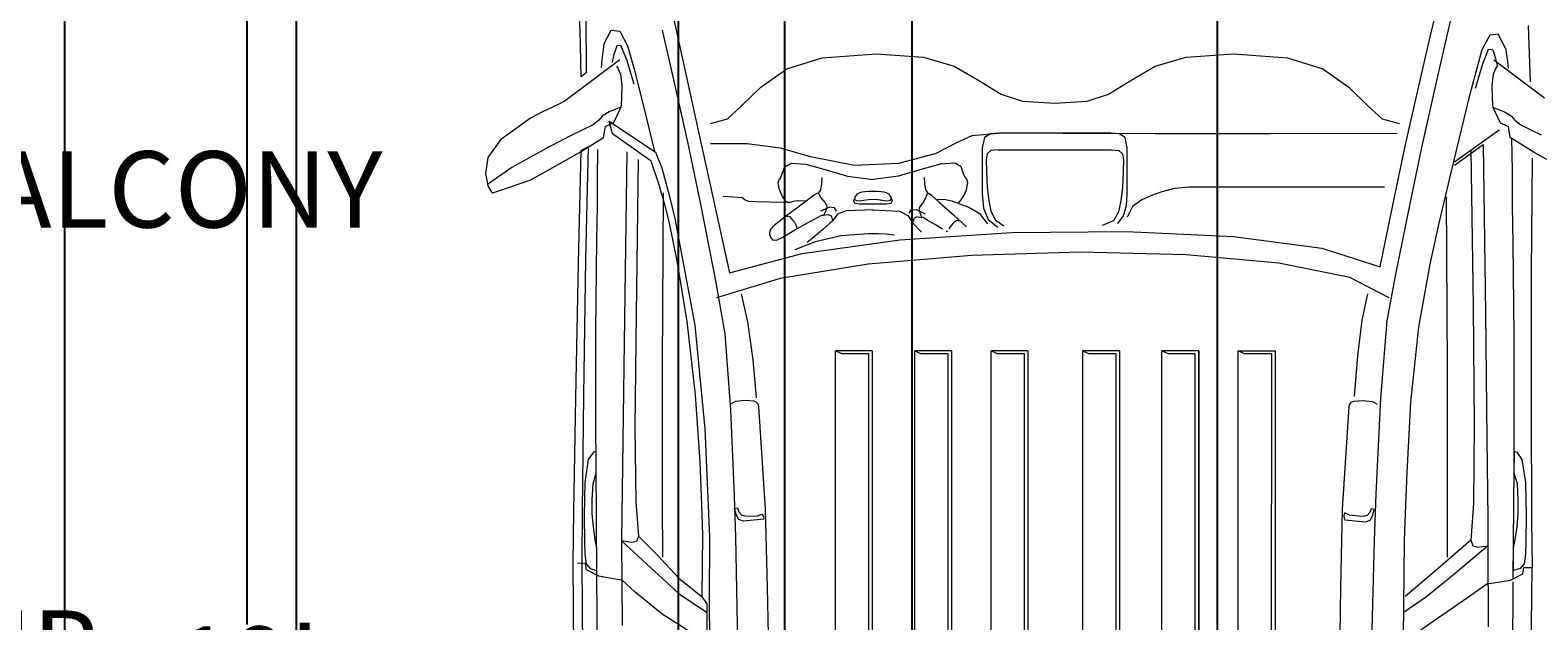
# Model space of a CAD drawing. Units: inches. Extents: x -36 to 401, y -686 to 73.
# Tile 5 of 15: x 184 to 303, y -532 to -485. Entities that reach past the tile are written whole.
import ezdxf

# ---------------------------------------------------------------- set-up
doc = ezdxf.new("R2010")
doc.units = ezdxf.units.IN
doc.header["$MEASUREMENT"] = 0
for name, color, linetype, lineweight in [('A-ANNO-DIMS', 2, 'Continuous', 18), ('A-ANNO-TEXT', 7, 'Continuous', 18), ('A-AREA-IDEN', 7, 'Continuous', 18), ('C-PKNG-VEHI', 8, 'Continuous', 13)]:
    doc.layers.add(name, color=color, linetype=linetype, lineweight=lineweight)
doc.styles.get("Standard").update_dxf_attribs({"font": 'arial.ttf'})
doc.dimstyles.get("Standard").update_dxf_attribs({"dimtxt": 0.18, "dimasz": 0.18, "dimexe": 0.18, "dimexo": 0.0625, "dimgap": 0.09, "dimtad": 0, "dimtih": 1, "dimtoh": 1, "dimdec": 0, "dimzin": 0, "dimdsep": 46, "dimlunit": 3, "dimtxsty": 'Standard', "dimcen": 0.09, "dimadec": 0, "dimazin": 0, "dimtfac": 1, "dimtdec": 0, "dimtofl": 0, "dimtmove": 0, "dimatfit": 3, "dimfxl": 1, "dimtolj": 1, "dimtzin": 0, "dimarcsym": 0})

# ---------------------------------------------------------------- blocks, each defined once
blk = doc.blocks.new('*D3')
at = {"layer": 'A-ANNO-DIMS', "color": 0, "lineweight": -2, "transparency": 16777216}
for p, q in [((200.9, -421.21), (201.62, -421.21)), ((201.44, -421.39), (201.44, -532.06)), ((201.44, -649.03), (201.44, -538.36)), ((200.9, -649.21), (201.62, -649.21))]:
    blk.add_line(p, q, dxfattribs=at)
at = {"layer": 'A-ANNO-DIMS', "color": 0, "transparency": 16777216}
for points in [[(201.41, -421.39), (201.47, -421.39), (201.44, -421.21)], [(201.41, -649.03), (201.47, -649.03), (201.44, -649.21)]]:
    blk.add_solid(points, dxfattribs=at)
at = {"layer": 'Defpoints', "color": 0, "transparency": 16777216}
for p in [(200.84, -421.21), (200.84, -649.21), (201.44, -649.21)]:
    blk.add_point(p, dxfattribs=at)
at = {"layer": 'A-ANNO-DIMS', "color": 0, "transparency": 16777216, "insert": (201.44, -535.21), "char_height": 6, "attachment_point": 5}
blk.add_mtext("\\A1;19'", dxfattribs=at)
blk = doc.blocks.new('*D73')
at = {"layer": 'A-ANNO-DIMS', "color": 0, "lineweight": -2, "transparency": 16777216}
for p, q in [((177.19, -421.27), (177.19, -685.69)), ((253.69, -421.27), (253.69, -685.69)), ((177.37, -685.51), (214.9, -685.51)), ((253.51, -685.51), (215.98, -685.51))]:
    blk.add_line(p, q, dxfattribs=at)
at = {"layer": 'A-ANNO-DIMS', "color": 0, "transparency": 16777216}
for points in [[(177.37, -685.48), (177.37, -685.54), (177.19, -685.51)], [(253.51, -685.48), (253.51, -685.54), (253.69, -685.51)]]:
    blk.add_solid(points, dxfattribs=at)
at = {"layer": 'Defpoints', "color": 0, "transparency": 16777216}
for p in [(177.19, -421.21), (253.69, -421.21), (253.69, -685.51)]:
    blk.add_point(p, dxfattribs=at)
at = {"layer": 'A-ANNO-DIMS', "color": 0, "transparency": 16777216, "insert": (215.44, -685.51), "char_height": 0.18, "attachment_point": 5}
blk.add_mtext('\\A1;6\'-4 1/2"', dxfattribs=at)
blk = doc.blocks.new('*D74')
at = {"layer": 'A-ANNO-DIMS', "color": 0, "lineweight": -2, "transparency": 16777216}
for p, q in [((277.69, -412.27), (277.69, -685.69)), ((313.69, -421.27), (313.69, -685.69)), ((277.87, -685.51), (295.36, -685.51)), ((313.51, -685.51), (296.02, -685.51))]:
    blk.add_line(p, q, dxfattribs=at)
at = {"layer": 'A-ANNO-DIMS', "color": 0, "transparency": 16777216}
for points in [[(277.87, -685.48), (277.87, -685.54), (277.69, -685.51)], [(313.51, -685.48), (313.51, -685.54), (313.69, -685.51)]]:
    blk.add_solid(points, dxfattribs=at)
at = {"layer": 'Defpoints', "color": 0, "transparency": 16777216}
for p in [(277.69, -412.21), (313.69, -421.21), (313.69, -685.51)]:
    blk.add_point(p, dxfattribs=at)
at = {"layer": 'A-ANNO-DIMS', "color": 0, "transparency": 16777216, "insert": (295.69, -685.51), "char_height": 0.18, "attachment_point": 5}
blk.add_mtext('\\A1;3\'-0"', dxfattribs=at)
blk = doc.blocks.new('*D87')
at = {"layer": 'A-ANNO-DIMS', "color": 0, "lineweight": -2, "transparency": 16777216}
for p, q in [((243.7, -154.81), (243.7, -685.69)), ((187.11, -163.6), (187.11, -685.69)), ((187.29, -685.51), (214.86, -685.51)), ((243.52, -685.51), (215.95, -685.51))]:
    blk.add_line(p, q, dxfattribs=at)
at = {"layer": 'A-ANNO-DIMS', "color": 0, "transparency": 16777216}
for points in [[(187.29, -685.48), (187.29, -685.54), (187.11, -685.51)], [(243.52, -685.48), (243.52, -685.54), (243.7, -685.51)]]:
    blk.add_solid(points, dxfattribs=at)
at = {"layer": 'Defpoints', "color": 0, "transparency": 16777216}
for p in [(243.7, -154.75), (187.11, -163.53), (243.7, -685.51)]:
    blk.add_point(p, dxfattribs=at)
at = {"layer": 'A-ANNO-DIMS', "color": 0, "transparency": 16777216, "insert": (215.4, -685.51), "char_height": 0.18, "attachment_point": 5}
blk.add_mtext('\\A1;4\'-8 1/2"', dxfattribs=at)
blk = doc.blocks.new('*D91')
at = {"layer": 'A-ANNO-DIMS', "color": 0, "lineweight": -2, "transparency": 16777216}
for p, q in [((205.32, -404.21), (205.32, -685.69)), ((235.34, -404.21), (235.34, -685.69)), ((205.5, -685.51), (220, -685.51)), ((235.16, -685.51), (220.66, -685.51))]:
    blk.add_line(p, q, dxfattribs=at)
at = {"layer": 'A-ANNO-DIMS', "color": 0, "transparency": 16777216}
for points in [[(205.5, -685.48), (205.5, -685.54), (205.32, -685.51)], [(235.16, -685.48), (235.16, -685.54), (235.34, -685.51)]]:
    blk.add_solid(points, dxfattribs=at)
at = {"layer": 'Defpoints', "color": 0, "transparency": 16777216}
for p in [(205.32, -404.14), (235.34, -404.14), (235.34, -685.51)]:
    blk.add_point(p, dxfattribs=at)
at = {"layer": 'A-ANNO-DIMS', "color": 0, "transparency": 16777216, "insert": (220.33, -685.51), "char_height": 0.18, "attachment_point": 5}
blk.add_mtext('\\A1;2\'-6"', dxfattribs=at)

msp = doc.modelspace()

# ---------------------------------------------------------------- linework, layer by layer
at = {"layer": 'C-PKNG-VEHI'}
for p, q in [((227.62, -485.32), (227.51, -482.83)), ((296.28, -483.48), (295.79, -485.61)), ((228.07, -484.2), (228.11, -488.65)), ((234.84, -483.75), (239.36, -504.4)), ((294.45, -485.83), (294.91, -483.89)), ((227.72, -488.98), (227.62, -485.32)), ((229.5, -486.4), (230.08, -485.31)), ((230.08, -485.31), (230.74, -485.39)), ((230.74, -485.39), (231.36, -486.54)), ((234.08, -485.3), (235.13, -489.89)), ((293.47, -490.06), (294.45, -485.83)), ((295.79, -485.61), (294.73, -490.2)), ((299.13, -485.7), (298.5, -486.85)), ((299.79, -485.61), (299.13, -485.7)), ((300.37, -486.71), (299.79, -485.61)), ((302.16, -484.94), (302.3, -489.38)), ((229.41, -487.01), (229.33, -487.64)), ((229.5, -486.4), (229.41, -487.01)), ((230.5, -486.54), (230.28, -487.23)), ((230.84, -486.5), (230.5, -486.54)), ((231.29, -487.65), (230.84, -486.5)), ((231.36, -486.54), (231.88, -488.37)), ((298.5, -486.85), (297.48, -490.66)), ((298.58, -487.95), (299.03, -486.8)), ((299.03, -486.8), (299.36, -486.85)), ((299.36, -486.85), (299.59, -487.54)), ((300.37, -486.71), (300.45, -487.24)), ((230.76, -487.64), (228.02, -489.69)), ((229.33, -487.64), (229.27, -488.27)), ((230.17, -487.68), (230.14, -487.84)), ((230.28, -487.23), (230.17, -487.68)), ((230.48, -488.14), (230.59, -488.3)), ((231.87, -489.56), (231.29, -487.65)), ((243.88, -488.35), (246.64, -487.47)), ((246.64, -487.47), (250.89, -487.17)), ((250.89, -487.17), (254.61, -487.42)), ((254.61, -487.42), (257.04, -488.14)), ((257.04, -488.14), (259.01, -489.28)), ((270.87, -489.28), (272.84, -488.14)), ((272.84, -488.14), (275.27, -487.42)), ((275.27, -487.42), (278.99, -487.17)), ((278.99, -487.17), (283.24, -487.47)), ((283.24, -487.47), (286, -488.35)), ((298, -489.87), (298.58, -487.95)), ((299.44, -487.64), (302.18, -489.69)), ((299.59, -487.54), (299.69, -487.98)), ((299.72, -488.14), (299.61, -488.3)), ((299.69, -487.98), (299.72, -488.14)), ((300.45, -487.24), (300.51, -487.78)), ((300.51, -487.78), (300.57, -488.33)), ((228.11, -488.65), (227.72, -488.98)), ((230.59, -488.3), (230.79, -488.78)), ((230.79, -488.78), (230.91, -489.65)), ((231.88, -488.37), (232.64, -491.39)), ((241.82, -489.78), (243.88, -488.35)), ((259.01, -489.28), (260.72, -490.33)), ((269.16, -490.33), (270.87, -489.28)), ((286, -488.35), (288.06, -489.78)), ((299.4, -488.78), (299.29, -489.65)), ((299.61, -488.3), (299.4, -488.78)), ((228.02, -489.69), (226.76, -490.64)), ((230.89, -490.58), (230.85, -491.17)), ((230.91, -489.65), (230.89, -490.58)), ((235.13, -489.89), (236.1, -494.23)), ((240.29, -491.28), (241.82, -489.78)), ((260.72, -490.33), (262.39, -490.89)), ((267.49, -490.89), (269.16, -490.33)), ((288.06, -489.78), (289.58, -491.28)), ((292.54, -494.2), (293.47, -490.06)), ((294.73, -490.2), (293.76, -494.53)), ((299.29, -489.65), (299.31, -490.58)), ((299.31, -490.58), (299.35, -491.17)), ((302.18, -489.69), (303.44, -490.64)), ((224.63, -491.76), (223.73, -492.24)), ((225.85, -491.17), (224.63, -491.76)), ((226.45, -490.87), (225.85, -491.17)), ((226.76, -490.64), (226.45, -490.87)), ((229.91, -491.73), (229.37, -492.07)), ((230.83, -491.37), (229.91, -491.73)), ((230.83, -491.37), (230.26, -492.6)), ((230.85, -491.17), (230.83, -491.37)), ((232.64, -491.39), (233.47, -494.86)), ((239.2, -492.29), (240.29, -491.28)), ((262.39, -490.89), (264.94, -491.05)), ((264.94, -491.05), (267.49, -490.89)), ((289.58, -491.28), (290.68, -492.29)), ((297.48, -490.66), (296.1, -496.4)), ((299.35, -491.17), (299.36, -491.37)), ((299.36, -491.37), (299.94, -492.6)), ((299.36, -491.37), (300.29, -491.73)), ((300.29, -491.73), (300.83, -492.07)), ((223.73, -492.24), (221.36, -493.94)), ((228.64, -492.74), (227.79, -493.17)), ((229.11, -492.38), (228.64, -492.74)), ((229.37, -492.07), (229.11, -492.38)), ((229.47, -493.74), (229.61, -492.88)), ((230.26, -492.6), (229.61, -492.88)), ((229.92, -492.46), (233.56, -494.9)), ((230.17, -493.46), (229.92, -492.46)), ((237.87, -492.64), (239.2, -492.29)), ((290.68, -492.29), (292.01, -492.64)), ((299.94, -492.6), (300.59, -492.88)), ((300.73, -493.74), (300.59, -492.88)), ((300.83, -492.07), (301.09, -492.38)), ((301.09, -492.38), (301.56, -492.74)), ((301.56, -492.74), (302.41, -493.17)), ((221.36, -493.94), (220.36, -495.32)), ((227.03, -493.53), (225.2, -494.48)), ((227.79, -493.17), (227.03, -493.53)), ((227.58, -494.92), (229.47, -493.74)), ((233.22, -495.6), (230.17, -493.46)), ((257.21, -494.18), (255.53, -495.04)), ((258.43, -493.61), (257.21, -494.18)), ((260.81, -493.41), (258.43, -493.61)), ((259.41, -493.74), (259.23, -494.56)), ((259.88, -493.45), (259.41, -493.74)), ((260.53, -493.42), (259.88, -493.45)), ((269.35, -493.42), (260.53, -493.42)), ((265.59, -493.44), (260.81, -493.41)), ((272.84, -493.45), (265.59, -493.44)), ((270, -493.45), (269.35, -493.42)), ((270.47, -493.74), (270, -493.45)), ((270.64, -494.56), (270.47, -493.74)), ((281.84, -493.45), (272.84, -493.45)), ((291.84, -493.43), (281.84, -493.45)), ((299.87, -493.17), (296.35, -495.68)), ((302.62, -494.92), (300.73, -493.74)), ((300.85, -493.78), (300.88, -496.4)), ((302.41, -493.17), (303.17, -493.53)), ((220.36, -495.32), (220.2, -496.59)), ((225.2, -494.48), (222.27, -496.12)), ((223.76, -497.07), (227.58, -494.92)), ((227.49, -503.64), (227.72, -494.76)), ((227.72, -494.76), (228.25, -494.45)), ((228.25, -494.45), (228.04, -503.37)), ((228.99, -494.7), (228.97, -497)), ((231.3, -494.88), (231.12, -507.99)), ((233.56, -494.9), (234.05, -496.14)), ((236.1, -494.23), (237.12, -499.13)), ((240.75, -494.26), (237.87, -494.26)), ((243.38, -494.6), (240.75, -494.26)), ((245.74, -495.26), (243.38, -494.6)), ((249.19, -495.96), (245.74, -495.26)), ((255.53, -495.04), (252.65, -495.79)), ((259.23, -494.56), (259.23, -498.18)), ((259.62, -495.04), (259.55, -495.5)), ((259.91, -494.78), (259.62, -495.04)), ((260.49, -494.71), (259.91, -494.78)), ((260.49, -494.71), (269.39, -494.71)), ((269.39, -494.71), (269.97, -494.78)), ((269.97, -494.78), (270.26, -495.04)), ((270.26, -495.04), (270.33, -495.5)), ((270.64, -498.18), (270.64, -494.56)), ((291.81, -497.67), (292.54, -494.2)), ((293.76, -494.53), (292.81, -499.1)), ((296.36, -495.93), (298.61, -494.3)), ((297.64, -494.75), (297.82, -507.04)), ((298.61, -494.3), (298.79, -507.56)), ((306.44, -497.07), (302.62, -494.92)), ((222.27, -496.12), (220.34, -497.45)), ((232.19, -495.49), (232.02, -507.62)), ((233.81, -497.39), (233.22, -495.6)), ((234.05, -496.14), (234.65, -498.4)), ((243.52, -496.61), (243.71, -496.05)), ((243.71, -496.05), (244.21, -495.76)), ((244.21, -495.76), (245.37, -495.84)), ((245.37, -495.84), (246.96, -496.28)), ((246.96, -496.28), (248.65, -496.8)), ((252.65, -495.79), (249.19, -495.96)), ((254.34, -496.28), (252.64, -496.8)), ((255.93, -495.84), (254.34, -496.28)), ((257.09, -495.76), (255.93, -495.84)), ((257.59, -496.05), (257.09, -495.76)), ((257.77, -496.61), (257.59, -496.05)), ((259.55, -495.5), (259.57, -496.42)), ((259.57, -496.42), (259.63, -497.65)), ((270.31, -496.42), (270.25, -497.65)), ((270.33, -495.5), (270.31, -496.42)), ((296.1, -496.4), (295.13, -500.49)), ((300.88, -496.4), (300.9, -499.16)), ((302.47, -495.38), (302.37, -504.35)), ((220.2, -496.59), (220.38, -497.56)), ((220.38, -497.56), (220.64, -498)), ((220.77, -498.1), (223.76, -497.07)), ((228.97, -497), (228.96, -499.15)), ((234.3, -499.12), (233.81, -497.39)), ((243.2, -497.31), (243.27, -497.02)), ((243.29, -497.87), (243.2, -497.31)), ((243.27, -497.02), (243.38, -496.96)), ((243.38, -496.96), (243.52, -496.61)), ((246.6, -497.39), (246.52, -497.86)), ((246.62, -496.89), (246.6, -497.39)), ((248.65, -496.8), (250.65, -497.05)), ((252.64, -496.8), (250.65, -497.05)), ((254.67, -496.89), (254.7, -497.38)), ((254.7, -497.38), (254.78, -497.86)), ((257.91, -496.96), (257.77, -496.61)), ((258.02, -497.02), (257.91, -496.96)), ((258, -497.87), (258.09, -497.31)), ((258.09, -497.31), (258.02, -497.02)), ((259.63, -497.65), (259.75, -498.74)), ((270.25, -497.65), (270.13, -498.74)), ((275.5, -497.66), (274.35, -497.77)), ((290.85, -497.66), (275.5, -497.66)), ((290.94, -501.87), (291.81, -497.67)), ((220.64, -498), (220.77, -498.1)), ((234.16, -498.1), (234.08, -511.66)), ((234.65, -498.4), (235.06, -500.11)), ((240.4, -498.49), (238.87, -498.38)), ((240.44, -498.55), (240.4, -498.49)), ((240.6, -498.67), (240.44, -498.55)), ((240.9, -498.77), (240.6, -498.67)), ((241.49, -498.81), (240.9, -498.77)), ((242.54, -498.84), (241.49, -498.81)), ((244.15, -498.85), (242.54, -498.84)), ((243.51, -498.34), (243.29, -497.87)), ((243.72, -498.66), (243.51, -498.34)), ((243.86, -498.82), (243.72, -498.66)), ((245.18, -498.92), (243.74, -499.98)), ((243.99, -498.88), (243.86, -498.82)), ((244.15, -498.85), (243.99, -498.88)), ((244.37, -498.77), (244.15, -498.85)), ((244.74, -498.73), (244.37, -498.77)), ((245.31, -498.75), (244.74, -498.73)), ((246.05, -498.27), (245.18, -498.92)), ((246.23, -498.16), (246.05, -498.27)), ((246.3, -498.16), (246.23, -498.16)), ((246.31, -498.18), (246.3, -498.16)), ((246.52, -497.86), (246.31, -498.18)), ((246.39, -498.18), (246.52, -498.46)), ((246.52, -498.46), (246.7, -498.69)), ((246.7, -498.69), (246.89, -498.89)), ((246.89, -498.89), (247, -499.08)), ((249.14, -498.74), (249.24, -498.44)), ((249.23, -498.93), (249.14, -498.74)), ((249.23, -498.59), (249.24, -498.44)), ((249.34, -498.73), (249.23, -498.59)), ((249.58, -498.99), (249.23, -498.93)), ((249.24, -498.44), (249.42, -498.19)), ((249.58, -498.75), (249.34, -498.73)), ((249.42, -498.19), (249.61, -498.08)), ((249.91, -498.7), (249.58, -498.75)), ((249.61, -498.08), (249.8, -498.03)), ((249.8, -498.03), (250.03, -498)), ((250.29, -498.65), (249.91, -498.7)), ((250.03, -498), (250.33, -497.98)), ((250.66, -498.62), (250.29, -498.65)), ((250.33, -497.98), (250.65, -497.98)), ((250.65, -497.98), (250.97, -497.98)), ((251.03, -498.65), (250.66, -498.62)), ((250.97, -497.98), (251.26, -498)), ((251.39, -498.7), (251.03, -498.65)), ((251.26, -498), (251.5, -498.03)), ((251.72, -498.75), (251.39, -498.7)), ((251.5, -498.03), (251.68, -498.08)), ((251.68, -498.08), (251.87, -498.19)), ((251.95, -498.73), (251.72, -498.75)), ((252.06, -498.93), (251.72, -498.99)), ((251.87, -498.19), (252.05, -498.44)), ((252.06, -498.59), (251.95, -498.73)), ((252.05, -498.44), (252.15, -498.74)), ((252.05, -498.44), (252.06, -498.59)), ((252.15, -498.74), (252.06, -498.93)), ((254.6, -498.84), (254.41, -499.09)), ((254.77, -498.51), (254.6, -498.84)), ((254.91, -498.18), (254.77, -498.51)), ((254.78, -497.86), (254.99, -498.18)), ((254.99, -498.18), (255, -498.16)), ((255, -498.16), (255.07, -498.16)), ((255.07, -498.16), (255.24, -498.29)), ((255.24, -498.29), (255.88, -498.85)), ((255.72, -498.61), (256.36, -498.62)), ((255.88, -498.85), (256.98, -499.84)), ((256.36, -498.62), (256.85, -498.73)), ((256.85, -498.73), (257.15, -498.85)), ((257.15, -498.85), (257.31, -498.88)), ((257.31, -498.88), (257.44, -498.82)), ((257.44, -498.82), (257.57, -498.66)), ((257.57, -498.66), (257.78, -498.34)), ((257.78, -498.34), (258, -497.87)), ((259.23, -498.18), (259.33, -499.3)), ((259.75, -498.74), (259.92, -499.51)), ((270.13, -498.74), (269.95, -499.59)), ((270.58, -499.11), (270.64, -498.18)), ((271.77, -498.66), (271.04, -499.18)), ((272.55, -498.32), (271.77, -498.66)), ((273.36, -498.03), (272.55, -498.32)), ((274.35, -497.77), (273.36, -498.03)), ((295.7, -498.41), (295.79, -511.89)), ((228.96, -499.15), (228.92, -501.77)), ((234.62, -500.35), (234.3, -499.12)), ((235.06, -500.11), (236.64, -508.5)), ((237.12, -499.13), (238.29, -505.15)), ((243.74, -499.98), (242.74, -500.78)), ((243.8, -499.97), (243.94, -499.93)), ((243.94, -499.93), (244.09, -499.97)), ((244.09, -499.97), (244.27, -500.16)), ((245.73, -500.32), (246.67, -499.84)), ((247.25, -499.22), (246.52, -499.54)), ((246.67, -499.84), (246.7, -499.85)), ((246.7, -499.85), (246.79, -499.86)), ((246.79, -499.86), (246.95, -499.84)), ((246.85, -499.68), (246.82, -499.79)), ((246.82, -499.79), (246.82, -499.83)), ((246.93, -499.48), (246.85, -499.68)), ((247.01, -499.27), (246.93, -499.48)), ((246.95, -499.84), (247.16, -499.81)), ((247, -499.08), (247.01, -499.27)), ((247.16, -499.81), (247.36, -499.92)), ((247.63, -499.27), (247.25, -499.22)), ((247.36, -499.92), (247.48, -500.27)), ((247.87, -499.78), (247.48, -500.27)), ((247.78, -499.55), (247.63, -499.27)), ((248.55, -499.52), (247.87, -499.78)), ((250.7, -499.44), (248.55, -499.52)), ((251.72, -498.99), (249.58, -498.99)), ((250.59, -499.44), (252.73, -499.55)), ((252.73, -499.55), (253.39, -499.89)), ((253.39, -499.89), (253.75, -500.43)), ((253.49, -499.7), (253.65, -499.43)), ((253.65, -499.43), (254.03, -499.4)), ((253.89, -500.09), (253.75, -500.43)), ((254.09, -499.99), (253.89, -500.09)), ((254.03, -499.4), (254.75, -499.75)), ((254.3, -500.03), (254.09, -499.99)), ((254.29, -499.27), (254.27, -499.46)), ((254.27, -499.46), (254.34, -499.68)), ((254.41, -499.09), (254.29, -499.27)), ((254.46, -500.06), (254.3, -500.03)), ((254.34, -499.68), (254.41, -499.87)), ((254.41, -499.87), (254.43, -499.99)), ((254.43, -499.99), (254.43, -500.03)), ((254.55, -500.05), (254.46, -500.06)), ((254.58, -500.05), (254.55, -500.05)), ((254.97, -500.27), (254.58, -500.05)), ((256.98, -499.84), (257.99, -500.77)), ((257.36, -498.93), (258.17, -499.23)), ((258.17, -499.23), (258.99, -499.7)), ((258.99, -499.7), (259.64, -500.55)), ((259.33, -499.3), (259.7, -500.21)), ((259.92, -499.51), (260.25, -500.22)), ((269.95, -499.59), (269.55, -500.31)), ((269.89, -500.51), (270.35, -499.9)), ((270.35, -499.9), (270.58, -499.11)), ((271.04, -499.18), (270.63, -500.02)), ((292.81, -499.1), (291.73, -504.49)), ((300.9, -499.16), (300.94, -502.07)), ((235.26, -503.46), (234.62, -500.35)), ((242.54, -501.07), (242.5, -501.35)), ((242.74, -500.78), (242.54, -501.07)), ((243.57, -501.58), (244.51, -501)), ((244.27, -500.16), (244.47, -500.42)), ((244.47, -500.42), (244.62, -500.67)), ((244.51, -501), (245.73, -500.32)), ((244.62, -500.67), (244.66, -500.9)), ((246.68, -501), (245.86, -501.7)), ((247.48, -500.27), (246.68, -501)), ((252.77, -501.81), (261.55, -501.23)), ((253.75, -500.43), (253.96, -500.67)), ((253.96, -500.67), (254.19, -500.92)), ((254.19, -500.92), (254.45, -501.2)), ((255.5, -500.58), (254.97, -500.27)), ((256.11, -500.96), (255.5, -500.58)), ((256.41, -501.13), (256.51, -501.12)), ((256.44, -501.13), (256.41, -501.13)), ((256.48, -501.13), (256.44, -501.13)), ((256.51, -501.12), (256.48, -501.13)), ((256.7, -500.8), (256.6, -500.95)), ((256.82, -500.65), (256.7, -500.8)), ((256.96, -500.49), (256.82, -500.65)), ((257.15, -500.32), (256.96, -500.49)), ((257.3, -500.28), (257.15, -500.32)), ((257.44, -500.32), (257.3, -500.28)), ((259.7, -500.21), (260.46, -500.81)), ((260.25, -500.22), (260.93, -500.69)), ((261.55, -501.23), (270.57, -501.13)), ((269.55, -500.31), (268.65, -500.68)), ((270.57, -501.13), (278.98, -501.54)), ((295.13, -500.49), (294.41, -503.71)), ((228.92, -501.77), (228.84, -509.04)), ((242.5, -501.35), (242.58, -501.6)), ((242.58, -501.6), (242.76, -501.8)), ((242.76, -501.8), (243.07, -501.83)), ((243.07, -501.83), (243.57, -501.58)), ((244.52, -502.57), (246.13, -501.93)), ((245.09, -502.87), (252.77, -501.81)), ((245.86, -501.7), (245.48, -502.02)), ((246.13, -501.93), (248.12, -501.47)), ((248.12, -501.47), (250.33, -501.3)), ((250.33, -501.3), (251.05, -501.3)), ((251.05, -501.3), (251.68, -501.33)), ((251.68, -501.33), (252.34, -501.41)), ((278.98, -501.54), (285.92, -502.46)), ((285.92, -502.46), (290.52, -503.91)), ((290.52, -503.91), (290.94, -501.87)), ((300.94, -502.07), (301.03, -509.35)), ((227.28, -514.2), (227.49, -503.64)), ((228.04, -503.37), (227.88, -514.04)), ((236.03, -508.21), (235.26, -503.46)), ((239.36, -504.4), (245.09, -502.87)), ((258.38, -503.03), (250.27, -503.71)), ((266.96, -502.78), (258.38, -503.03)), ((275.26, -502.98), (266.96, -502.78)), ((282.56, -503.63), (275.26, -502.98)), ((288.12, -504.75), (282.56, -503.63)), ((243.35, -504.83), (238.35, -506.35)), ((250.27, -503.71), (243.35, -504.83)), ((291.22, -506.35), (288.12, -504.75)), ((291.73, -504.49), (291.05, -508.18)), ((294.41, -503.71), (293.53, -508.67)), ((302.37, -504.35), (302.38, -514.97)), ((238.29, -505.15), (238.99, -509.18)), ((240.29, -506.05), (240.78, -508.26)), ((289.53, -506.05), (289.07, -508.12)), ((297.82, -507.04), (297.91, -516.35)), ((231.12, -507.99), (230.99, -517.58)), ((232.02, -507.62), (231.94, -516.57)), ((236.7, -513.98), (236.03, -508.21)), ((240.78, -508.26), (241.19, -511.23)), ((289.07, -508.12), (288.72, -510.92)), ((291.05, -508.18), (290.54, -514.26)), ((298.79, -507.56), (298.91, -517.49)), ((228.84, -509.04), (228.84, -516.24)), ((236.64, -508.5), (237.44, -516.67)), ((238.99, -509.18), (239.44, -515.16)), ((293.53, -508.67), (292.9, -514.57)), ((301.03, -509.35), (301.03, -516.55)), ((247.7, -586.39), (247.7, -510.52)), ((248.19, -510.76), (247.7, -510.52)), ((250.59, -510.52), (247.7, -510.52)), ((250.33, -510.76), (248.19, -510.76)), ((250.3, -585.18), (250.33, -510.76)), ((250.59, -510.52), (250.59, -586.39)), ((250.59, -510.52), (250.59, -586.39)), ((253.93, -586.39), (253.93, -510.52)), ((254.42, -510.76), (253.93, -510.52)), ((256.82, -510.52), (253.93, -510.52)), ((256.56, -510.76), (254.42, -510.76)), ((256.53, -585.18), (256.56, -510.76)), ((256.82, -510.52), (256.82, -586.39)), ((256.82, -510.52), (256.82, -586.39)), ((259.94, -586.39), (259.94, -510.52)), ((260.43, -510.76), (259.94, -510.52)), ((262.83, -510.52), (259.94, -510.52)), ((262.57, -510.76), (260.43, -510.76)), ((262.54, -585.18), (262.57, -510.76)), ((262.83, -510.52), (262.83, -586.39)), ((262.83, -510.52), (262.83, -586.39)), ((267.61, -510.76), (267.12, -510.52)), ((270.02, -510.52), (267.12, -510.52)), ((267.13, -586.39), (267.13, -510.52)), ((269.76, -510.76), (267.61, -510.76)), ((269.73, -585.18), (269.76, -510.76)), ((270.02, -510.52), (270.02, -586.39)), ((270.02, -510.52), (270.02, -586.39)), ((273.84, -510.76), (273.35, -510.52)), ((276.25, -510.52), (273.35, -510.52)), ((273.36, -586.39), (273.36, -510.52)), ((275.98, -510.76), (273.84, -510.76)), ((275.96, -585.18), (275.98, -510.76)), ((276.24, -510.52), (276.24, -586.39)), ((276.25, -510.52), (276.25, -586.39)), ((279.36, -586.39), (279.36, -510.52)), ((279.85, -510.76), (279.36, -510.52)), ((279.36, -510.52), (282.25, -510.52)), ((281.99, -510.76), (279.85, -510.76)), ((281.97, -585.18), (281.99, -510.76)), ((282.25, -510.52), (282.25, -586.39)), ((234.08, -511.66), (234.07, -522.4)), ((241.19, -511.23), (241.46, -514.23)), ((288.72, -510.92), (288.46, -514.12)), ((295.79, -511.89), (295.79, -522.48)), ((227.14, -523.17), (227.28, -514.2)), ((227.88, -514.04), (227.78, -523.12)), ((237.06, -519.26), (236.7, -513.98)), ((290.54, -514.26), (290.17, -521.79)), ((239.44, -515.16), (239.73, -521.94)), ((239.85, -514.51), (239.45, -514.73)), ((240.61, -514.43), (239.85, -514.51)), ((241.3, -514.49), (240.61, -514.43)), ((241.47, -514.58), (241.3, -514.49)), ((241.62, -514.72), (241.47, -514.58)), ((241.68, -514.9), (241.62, -514.72)), ((242.2, -522.99), (241.68, -514.9)), ((287.56, -522.99), (288.07, -514.9)), ((288.07, -514.9), (288.13, -514.72)), ((288.13, -514.72), (288.27, -514.58)), ((288.27, -514.58), (288.45, -514.49)), ((288.45, -514.49), (289.13, -514.43)), ((289.13, -514.43), (289.9, -514.51)), ((289.9, -514.51), (290.29, -514.73)), ((292.9, -514.57), (292.61, -520.11)), ((302.38, -514.97), (302.42, -523.85)), ((228.84, -516.24), (228.85, -519.5)), ((231.94, -516.57), (232, -522.38)), ((237.44, -516.67), (237.8, -525.17)), ((297.91, -516.35), (297.86, -522.53)), ((301.03, -516.55), (301.02, -519.81)), ((230.99, -517.58), (230.91, -523.46)), ((298.91, -517.49), (298.97, -523.71)), ((228.67, -518.5), (228.27, -519.08)), ((228.88, -518.46), (228.67, -518.5)), ((228.9, -520.15), (228.88, -518.46)), ((301.04, -520.15), (301.06, -518.46)), ((301.06, -518.46), (301.26, -518.5)), ((301.26, -518.5), (301.66, -519.08)), ((228.27, -519.08), (227.99, -520.89)), ((228.64, -520.98), (228.9, -520.15)), ((228.85, -519.5), (228.92, -528.19)), ((237.22, -523.35), (237.06, -519.26)), ((292.61, -520.11), (292.45, -524.01)), ((301.02, -519.81), (300.94, -528.5)), ((301.3, -520.98), (301.04, -520.15)), ((301.66, -519.08), (301.94, -520.89)), ((227.99, -520.89), (227.94, -523.48)), ((228.57, -522.21), (228.64, -520.98)), ((301.37, -522.21), (301.3, -520.98)), ((301.94, -520.89), (301.99, -523.48)), ((228.57, -523.32), (228.57, -522.21)), ((232, -522.38), (232.22, -525.1)), ((234.07, -522.4), (234.09, -526.77)), ((239.73, -521.94), (239.84, -525.17)), ((290.17, -521.79), (290.03, -525.48)), ((295.79, -522.48), (295.77, -526.77)), ((297.86, -522.53), (297.64, -525.41)), ((301.36, -523.32), (301.37, -522.21)), ((227.08, -527.24), (227.14, -523.17)), ((227.78, -523.12), (227.75, -527.24)), ((227.94, -523.48), (227.97, -525.61)), ((228.67, -524.41), (228.57, -523.32)), ((230.91, -523.46), (230.89, -525.47)), ((237.26, -524.99), (237.22, -523.35)), ((239.76, -522.94), (240.01, -522.89)), ((239.88, -523.4), (239.76, -522.94)), ((240.09, -523.79), (239.88, -523.4)), ((240.01, -522.89), (240.11, -523.19)), ((240.47, -523.93), (240.09, -523.79)), ((240.11, -523.19), (240.31, -523.43)), ((240.31, -523.43), (240.61, -523.51)), ((242.08, -523.77), (240.47, -523.93)), ((240.61, -523.51), (240.95, -523.53)), ((240.95, -523.53), (241.58, -523.52)), ((241.58, -523.52), (241.92, -523.37)), ((241.92, -523.37), (242.04, -523.56)), ((242.04, -523.56), (242.08, -523.71)), ((242.08, -523.71), (242.08, -523.77)), ((242.36, -529.15), (242.2, -522.99)), ((287.43, -529.15), (287.56, -522.99)), ((287.73, -523.26), (287.65, -523.49)), ((287.65, -523.49), (287.69, -523.72)), ((287.69, -523.72), (287.73, -523.82)), ((288.11, -523.45), (287.73, -523.26)), ((288.82, -523.54), (288.11, -523.45)), ((289.2, -523.57), (288.82, -523.54)), ((289.5, -523.49), (289.2, -523.57)), ((289.7, -523.24), (289.5, -523.49)), ((289.8, -522.95), (289.7, -523.24)), ((289.72, -523.85), (289.94, -523.46)), ((290.05, -523), (289.8, -522.95)), ((289.94, -523.46), (290.05, -523)), ((298.97, -523.71), (298.98, -525.86)), ((301.27, -524.41), (301.36, -523.32)), ((301.99, -523.48), (301.97, -525.61)), ((228.84, -525.52), (228.67, -524.41)), ((237.21, -529.88), (237.26, -524.99)), ((287.73, -523.82), (289.35, -523.98)), ((289.35, -523.98), (289.72, -523.85)), ((292.45, -524.01), (292.4, -525.48)), ((301.1, -525.52), (301.27, -524.41)), ((302.42, -523.85), (302.45, -527.56)), ((227.97, -525.61), (228, -526.5)), ((228.93, -526.04), (228.84, -525.52)), ((228.93, -527.8), (228.93, -526.04)), ((230.89, -525.47), (233.15, -527.56)), ((231.67, -525.61), (230.89, -525.47)), ((230.89, -525.47), (230.92, -532.14)), ((232.07, -525.53), (231.67, -525.61)), ((232.22, -525.1), (232.07, -525.53)), ((232.22, -525.1), (233.66, -526.54)), ((237.8, -525.17), (237.77, -530.16)), ((239.84, -525.17), (240, -533.51)), ((290.03, -525.48), (289.82, -533.45)), ((292.4, -525.48), (292.33, -533.09)), ((297.64, -525.41), (295.26, -527.5)), ((298.98, -525.86), (296.56, -527.92)), ((297.64, -525.41), (297.8, -525.86)), ((297.8, -525.86), (298.2, -525.98)), ((298.2, -525.98), (298.98, -525.86)), ((298.98, -525.86), (299.01, -532.23)), ((301, -526.04), (301.1, -525.52)), ((301, -527.8), (301, -526.04)), ((301.97, -525.61), (301.94, -526.5)), ((227.14, -534.09), (227.08, -527.24)), ((228.06, -527.26), (227.41, -527.24)), ((227.75, -527.24), (227.81, -534.08)), ((228, -526.5), (228.11, -527.28)), ((228.13, -527.76), (228.06, -527.26)), ((228.11, -527.28), (228.41, -527.66)), ((233.66, -526.54), (235.41, -528.43)), ((301.83, -527.28), (301.53, -527.66)), ((301.94, -526.5), (301.83, -527.28)), ((229.09, -528.26), (228.13, -527.76)), ((228.41, -527.66), (228.93, -527.8)), ((228.92, -528.19), (228.98, -538.68)), ((230.24, -528.46), (229.09, -528.26)), ((230.92, -528.58), (230.24, -528.46)), ((233.15, -527.56), (235.43, -529.67)), ((235.41, -528.43), (237.21, -529.88)), ((295.26, -527.5), (293.29, -529.18)), ((296.56, -527.92), (294.16, -529.89)), ((300.76, -528.56), (301.73, -528.07)), ((301.53, -527.66), (301, -527.8)), ((301.73, -528.07), (301.81, -527.56)), ((301.81, -527.56), (302.43, -527.56)), ((302.39, -534.4), (302.45, -527.56)), ((231.96, -529.5), (230.92, -528.58)), ((234.07, -531.23), (231.96, -529.5)), ((235.43, -529.67), (237.62, -531.11)), ((242.43, -532.86), (242.36, -529.15)), ((287.38, -532.86), (287.43, -529.15)), ((293.29, -529.18), (292.48, -529.86)), ((297.45, -529.87), (298.91, -528.86)), ((298.91, -528.86), (299.6, -528.75)), ((299.6, -528.75), (300.76, -528.56)), ((300.95, -528.69), (300.9, -539.19)), ((237.61, -530.43), (237.21, -529.88)), ((237.63, -535.28), (237.61, -530.43)), ((237.77, -530.16), (237.8, -533.34)), ((294.16, -529.89), (292.4, -531.08)), ((294.95, -531.6), (297.45, -529.87)), ((236.31, -532.67), (234.07, -531.23)), ((293.63, -532.52), (294.95, -531.6))]:
    msp.add_line(p, q, dxfattribs=at)

# ---------------------------------------------------------------- texts
at = {"layer": 'A-ANNO-TEXT', "insert": (178.66, -530.94), "char_height": 6, "attachment_point": 1}
msp.add_mtext_dynamic_manual_height_columns('UP', width=0.1631, gutter_width=1, heights=[0], dxfattribs=at)
at = {"layer": 'A-AREA-IDEN', "insert": (133.95, -494.83), "char_height": 6, "attachment_point": 1}
msp.add_mtext('6\'-6" WIDE BALCONY', dxfattribs=at)

# ---------------------------------------------------------------- dimensions: what is measured, and where the dimension line sits
at = {"layer": 'A-ANNO-DIMS'}
for base, p1, p2, picture, middle in [((243.7, -685.51), (187.11, -163.53), (243.7, -154.75), '*D87', (215.4, -685.51)), ((235.34, -685.51), (205.32, -404.14), (235.34, -404.14), '*D91', (220.33, -685.51)), ((313.69, -685.51), (277.69, -412.21), (313.69, -421.21), '*D74', (295.69, -685.51)), ((253.69, -685.51), (177.19, -421.21), (253.69, -421.21), '*D73', (215.44, -685.51))]:
    dim = msp.add_linear_dim(base=base, p1=p1, p2=p2, dimstyle='Standard', override={"dimdec": 1, "dimlfac": 1, "dimrnd": 0, "dimzin": 1, "dimdsep": 46, "dimlunit": 4, "dimfrac": 2}, dxfattribs=at)
    dim.commit()
    dim.dimension.update_dxf_attribs({"geometry": picture, "text_midpoint": middle})
dim = msp.add_linear_dim(base=(201.44, -649.21), p1=(200.84, -421.21), p2=(200.84, -649.21), angle=90, dimstyle='Standard', override={"dimtxt": 6, "dimclrd": 0, "dimclre": 0, "dimclrt": 0}, dxfattribs=at)
dim.commit()
dim.dimension.update_dxf_attribs({"geometry": '*D3', "text_midpoint": (201.44, -535.21)})

doc.saveas('drawing.dxf')
